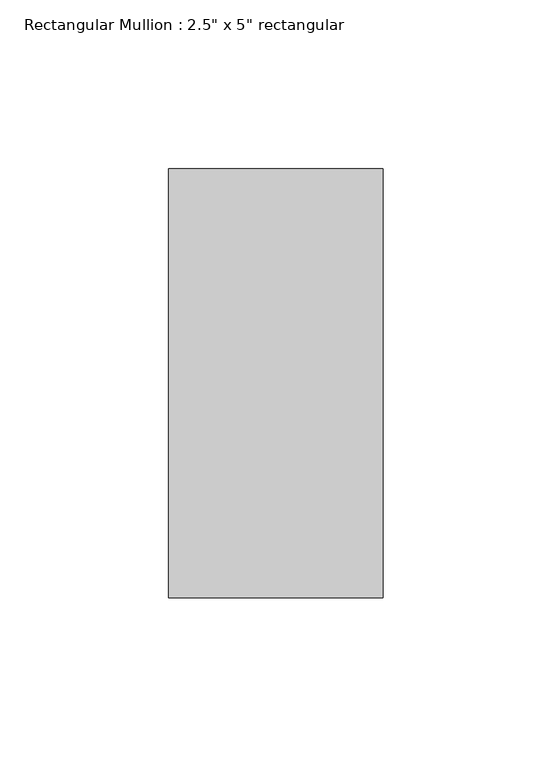
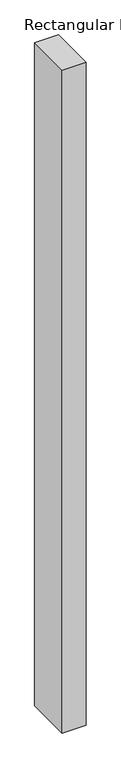
"""IFC4 building model written with IfcOpenShell, lengths in millimetres: member geometry."""

from ifc_helpers import new_model, si_unit, frame, origin, place, context, project, spatial, polyline, outline, extrude, source, transform, mapped, element, save


def member_780abd71(model_context):
    return source(origin(), model_context, "Body", "SweptSolid", [
        extrude(outline(polyline([(31.75, 63.5), (31.75, -63.5), (-31.75, -63.5), (-31.75, 63.5), (31.75, 63.5)])), frame((0.0, 0.0, -1868.0529055), z_axis=(0.0, 0.0, 1.0), x_axis=(1.0, 0.0, 0.0)), (0.0, 0.0, 1.0), 1868.0529055),
    ])


if __name__ == "__main__":
    model = new_model("IFC4")
    model_context = context("Model", 3, world=origin())
    ifc_project = project(units=[si_unit("LENGTHUNIT", "METRE", prefix="MILLI")], contexts=[model_context])
    site = spatial("IfcSite", under=ifc_project)
    building = spatial("IfcBuilding", under=site)
    placement = place(None, origin())
    member_shape = member_780abd71(model_context)
    element("IfcMember", 1, ObjectType="Rectangular Mullion : 2.5\" x 5\" rectangular", at=placement, inside=building, context=model_context, shape_type="MappedRepresentation", body=[
        mapped(member_shape, transform((0.0, 0.0, 0.0), x_axis=(1.0, 0.0, 0.0), y_axis=(0.0, 1.0, 0.0), z_axis=(0.0, 0.0, 1.0))),
    ])
    save(model, "model.ifc")

# Revit data of these elements
# Type "Rectangular Mullion : 2.5\" x 5\" rectangular"
#   built-in parameter 1007304 = 0.416667 (stored number, unit not read)
#   built-in parameter 1007301 = 0.104167 (stored number, unit not read)
#   built-in parameter 1007300 = 0.104167 (stored number, unit not read)
# Element 1 (IfcMember, "Rectangular Mullion : 2.5\" x 5\" rectangular")
#   Materials on its faces: "Aluminum"
# Materials
#   "Aluminum": class "Metal", colour RGB 247 247 247, transparency 0, Description = "Aluminum 6061", Cost = 0
